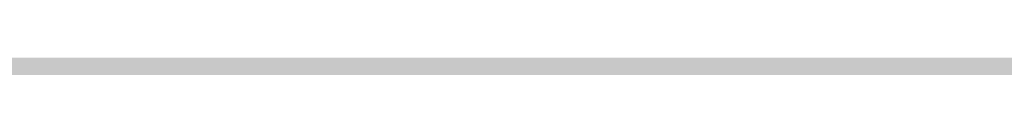
# Model space of a CAD drawing. Units: millimetres. Extents: x 0 to 2267, y 0 to 1823.
# Tile 206 of 256: x 1841.442 to 1842.748, y 1127.404 to 1127.414. Entities that reach past the tile are written whole.
import ezdxf

# ---------------------------------------------------------------- set-up
doc = ezdxf.new("R2010")
doc.units = ezdxf.units.MM
doc.header["$MEASUREMENT"] = 0
doc.layers.add('M-DIMS', color=2, linetype='Continuous', lineweight=25)
doc.layers.add('M-HATC', color=252, linetype='Continuous', lineweight=18)
doc.styles.get("Standard").update_dxf_attribs({"font": 'arial.ttf'})
doc.dimstyles.get("Standard").update_dxf_attribs({"dimtxt": 7, "dimasz": 4, "dimexe": 0.18, "dimexo": 0.0625, "dimgap": 0.09, "dimtad": 0, "dimdec": 0, "dimzin": 0, "dimdsep": 46, "dimtxsty": 'Standard', "dimcen": 0.09, "dimadec": 0, "dimazin": 0, "dimtfac": 1, "dimtdec": 0, "dimtofl": 0, "dimtmove": 0, "dimatfit": 3, "dimfxl": 1, "dimtolj": 1, "dimtzin": 0, "dimarcsym": 0})

# ---------------------------------------------------------------- blocks, each defined once
blk = doc.blocks.new('*D1')
at = {"layer": 'Defpoints', "color": 0, "transparency": 16777216}
for p in [(1593.4289, 1127.4171), (1843.4289, 1127.4171), (1843.4289, 955.6278)]:
    blk.add_point(p, dxfattribs=at)
at = {"layer": 'M-DIMS', "color": 0, "lineweight": -2, "transparency": 16777216}
for p, q in [((1593.4289, 1127.3546), (1593.4289, 955.4478)), ((1843.4289, 1127.3546), (1843.4289, 955.4478)), ((1597.4289, 955.6278), (1710.5582, 955.6278)), ((1839.4289, 955.6278), (1726.2996, 955.6278))]:
    blk.add_line(p, q, dxfattribs=at)
at = {"layer": 'M-DIMS', "color": 0, "transparency": 16777216}
for points in [[(1597.4289, 956.2944), (1597.4289, 954.9611), (1593.4289, 955.6278)], [(1839.4289, 956.2944), (1839.4289, 954.9611), (1843.4289, 955.6278)]]:
    blk.add_solid(points, dxfattribs=at)
at = {"layer": 'M-DIMS', "color": 0, "transparency": 16777216, "insert": (1718.4289, 955.6278), "char_height": 7, "attachment_point": 5}
blk.add_mtext('\\A1;250', dxfattribs=at)

msp = doc.modelspace()

# ---------------------------------------------------------------- hatches: boundary and pattern name
at = {"layer": 'M-HATC'}
h = msp.add_hatch(color=256, dxfattribs=at)
h.dxf.hatch_style = 1
h.paths.add_polyline_path([(2055.771, 1603.062), (1381.0868, 1603.062), (1381.0868, 1598.062), (2055.771, 1598.062)])
h.paths.add_polyline_path([(2055.771, 1598.062), (1381.0868, 1598.062), (1381.0868, 1593.062), (2055.771, 1593.062)])
h.paths.add_polyline_path([(2051.3074, 1536.7609), (1385.5504, 1536.7609), (1385.5504, 1526.7609), (1387.5504, 1526.7609), (1388.5366, 1525.0528), (1385.3319, 1521.2335), (1385.3319, 1521.2226), (2050.2542, 1522.7491), (2048.3212, 1525.0528), (2049.3074, 1526.7609), (2051.3074, 1526.7609)])
edge = h.paths.add_edge_path()
edge.add_arc((1847.5345, 1379.1492), 135, 222.603061, 222.890851, ccw=False)
edge.add_line((1748.1663, 1287.7656), (1683.0921, 1287.7656))
edge.add_arc((1583.7239, 1379.1492), 135, 317.109149, 317.396939, ccw=False)
edge.add_arc((1678.9686, 1290.6707), 5, 222.8909, 317.1091, ccw=False)
edge.add_arc((1774.2133, 1379.1492), 135, 222.603061, 222.890851, ccw=False)
edge.add_line((1674.8451, 1287.7656), (1609.7709, 1287.7656))
edge.add_arc((1510.4027, 1379.1492), 135, 317.109149, 317.396939, ccw=False)
edge.add_arc((1605.6474, 1290.6707), 5, 222.8909, 317.1091, ccw=False)
edge.add_arc((1700.8921, 1379.1492), 135, 222.603061, 222.890851, ccw=False)
edge.add_line((1601.5239, 1287.7656), (1536.4497, 1287.7656))
edge.add_arc((1437.0815, 1379.1492), 135, 317.109149, 317.396939, ccw=False)
edge.add_arc((1532.3262, 1290.6707), 5, 222.8909, 317.1091, ccw=False)
edge.add_arc((1627.5709, 1379.1492), 135, 222.603061, 222.890851, ccw=False)
edge.add_line((1528.2027, 1287.7656), (1505.9289, 1287.7656))
edge.add_spline(control_points=[(1505.9289, 1287.7656), (1504.2622, 1287.7656), (1504.2622, 1282.7656), (1505.9289, 1282.7656)], knot_values=[0, 0, 0, 0, 5, 5, 5, 5], degree=3, periodic=0)
edge.add_line((1505.9289, 1282.7656), (1930.9289, 1282.7656))
edge.add_spline(control_points=[(1930.9289, 1282.7656), (1932.5956, 1282.7656), (1932.5956, 1287.7656), (1930.9289, 1287.7656)], knot_values=[0, 0, 0, 0, 5, 5, 5, 5], degree=3, periodic=0)
edge.add_line((1930.9289, 1287.7656), (1903.0557, 1287.7656))
edge.add_arc((1803.6875, 1379.1492), 135, 317.109149, 317.396939, ccw=False)
edge.add_arc((1898.9322, 1290.6707), 5, 222.8909, 317.1091, ccw=False)
edge.add_arc((1994.1769, 1379.1492), 135, 222.603061, 222.890851, ccw=False)
edge.add_line((1894.8087, 1287.7656), (1829.7345, 1287.7656))
edge.add_arc((1730.3663, 1379.1492), 135, 317.109149, 317.396939, ccw=False)
edge.add_arc((1825.611, 1290.6707), 5, 222.8909, 317.1091, ccw=False)
edge.add_arc((1920.8557, 1379.1492), 135, 222.603061, 222.890851, ccw=False)
edge.add_line((1821.4875, 1287.7656), (1756.4133, 1287.7656))
edge.add_arc((1657.0451, 1379.1492), 135, 317.109149, 317.396939, ccw=False)
edge.add_arc((1752.2898, 1290.6707), 5, 222.8909, 317.1091, ccw=False)
edge = h.paths.add_edge_path()
edge.add_spline(control_points=[(1843.4289, 1227.2475), (1845.0956, 1227.2475), (1845.0956, 1232.2475), (1843.4289, 1232.2475)], knot_values=[0, 0, 0, 0, 5, 5, 5, 5], degree=3, periodic=0)
edge.add_line((1843.4289, 1232.2475), (1593.4289, 1232.2475))
edge.add_spline(control_points=[(1593.4289, 1232.2475), (1591.7622, 1232.2475), (1591.7622, 1227.2475), (1593.4289, 1227.2475)], knot_values=[0, 0, 0, 0, 5, 5, 5, 5], degree=3, periodic=0)
edge.add_line((1593.4289, 1227.2475), (1843.4289, 1227.2475))
h.paths.add_polyline_path([(1905.9289, 1127.4171), (1530.9289, 1127.4171, 0.414214), (1520.9289, 1117.4171), (1530.9289, 1117.4171), (1915.9289, 1117.4171, 0.414214)])
edge = h.paths.add_edge_path()
edge.add_arc((1397.0858, 1498.4078), 12.7299, 90.78215, 190.87871, ccw=False)
edge.add_line((1396.912, 1511.1365), (1428.0097, 1511.3488))
edge.add_line((1428.0097, 1511.3488), (1433.0097, 1511.3488))
edge.add_line((1433.0097, 1511.3488), (1434.439, 1511.3488))
edge.add_arc((1419.474, 1498.0804), 20, 41.561, 74.08211)
edge.add_line((1424.9592, 1517.3135), (1399.9351, 1517.2561))
edge.add_spline(control_points=[(1399.9307, 1517.2561), (1399.884, 1517.2131), (1399.8328, 1517.1689), (1399.7774, 1517.1236)], knot_values=[11.567499, 11.567499, 11.567499, 11.567499, 11.814249, 11.814249, 11.814249, 11.814249], degree=3, periodic=0)
edge.add_spline(control_points=[(1399.6328, 1517.0099), (1399.5831, 1516.9721), (1399.5307, 1516.9338), (1399.4759, 1516.8947)], knot_values=[11.167718, 11.167718, 11.167718, 11.167718, 11.365188, 11.365188, 11.365188, 11.365188], degree=3, periodic=0)
edge.add_spline(control_points=[(1399.3398, 1516.8001), (1399.1514, 1516.6719), (1398.9384, 1516.5377), (1398.704, 1516.3994)], knot_values=[10.376405, 10.376405, 10.376405, 10.376405, 11.00994, 11.00994, 11.00994, 11.00994], degree=3, periodic=0)
edge.add_spline(control_points=[(1398.6572, 1516.3719), (1398.5789, 1516.326), (1398.4983, 1516.2797), (1398.4155, 1516.2331)], knot_values=[10.125175, 10.125175, 10.125175, 10.125175, 10.334406, 10.334406, 10.334406, 10.334406], degree=3, periodic=0)
edge.add_spline(control_points=[(1398.2642, 1516.1487), (1398.196, 1516.1111), (1398.1263, 1516.0732), (1398.0555, 1516.0351)], knot_values=[9.832246, 9.832246, 9.832246, 9.832246, 9.999658, 9.999658, 9.999658, 9.999658], degree=3, periodic=0)
edge.add_spline(control_points=[(1397.9987, 1516.0048), (1397.7312, 1515.8621), (1397.446, 1515.7171), (1397.1466, 1515.5714)], knot_values=[9.161808, 9.161808, 9.161808, 9.161808, 9.787769, 9.787769, 9.787769, 9.787769], degree=3, periodic=0)
edge.add_spline(control_points=[(1397.1466, 1515.5714), (1396.8418, 1515.423), (1396.5222, 1515.274), (1396.1914, 1515.1262)], knot_values=[8.524455, 8.524455, 8.524455, 8.524455, 9.161808, 9.161808, 9.161808, 9.161808], degree=3, periodic=0)
edge.add_spline(control_points=[(1396.0777, 1515.0756), (1395.9854, 1515.0348), (1395.8922, 1514.994), (1395.7983, 1514.9534)], knot_values=[8.275193, 8.275193, 8.275193, 8.275193, 8.451726, 8.451726, 8.451726, 8.451726], degree=3, periodic=0)
edge.add_spline(control_points=[(1395.6018, 1514.8691), (1395.4997, 1514.8257), (1395.3968, 1514.7824), (1395.2932, 1514.7394)], knot_values=[7.962917, 7.962917, 7.962917, 7.962917, 8.152764, 8.152764, 8.152764, 8.152764], degree=3, periodic=0)
edge.add_spline(control_points=[(1395.2116, 1514.7057), (1394.8278, 1514.5475), (1394.4345, 1514.3929), (1394.0364, 1514.2442)], knot_values=[7.21254, 7.21254, 7.21254, 7.21254, 7.913148, 7.913148, 7.913148, 7.913148], degree=3, periodic=0)
edge.add_spline(control_points=[(1394.0364, 1514.2442), (1393.7076, 1514.1214), (1393.3754, 1514.0027), (1393.0427, 1513.8895)], knot_values=[6.633733, 6.633733, 6.633733, 6.633733, 7.21254, 7.21254, 7.21254, 7.21254], degree=3, periodic=0)
edge.add_spline(control_points=[(1392.8214, 1513.815), (1392.7198, 1513.7812), (1392.6181, 1513.7479), (1392.5166, 1513.7152)], knot_values=[6.328796, 6.328796, 6.328796, 6.328796, 6.505493, 6.505493, 6.505493, 6.505493], degree=3, periodic=0)
edge.add_spline(control_points=[(1392.5166, 1513.7152), (1392.3187, 1513.6515), (1392.1212, 1513.59), (1391.9244, 1513.531)], knot_values=[5.984605, 5.984605, 5.984605, 5.984605, 6.328796, 6.328796, 6.328796, 6.328796], degree=3, periodic=0)
edge.add_spline(control_points=[(1391.7915, 1513.4915), (1391.3122, 1513.3501), (1390.8384, 1513.2239), (1390.3784, 1513.1171)], knot_values=[5.066697, 5.066697, 5.066697, 5.066697, 5.907055, 5.907055, 5.907055, 5.907055], degree=3, periodic=0)
edge.add_spline(control_points=[(1390.3784, 1513.1171), (1390.1797, 1513.071), (1389.9836, 1513.0284), (1389.7907, 1512.9899)], knot_values=[4.70367, 4.70367, 4.70367, 4.70367, 5.066695, 5.066695, 5.066695, 5.066695], degree=3, periodic=0)
edge.add_spline(control_points=[(1389.422, 1512.9204), (1389.2459, 1512.8892), (1389.0729, 1512.8617), (1388.9036, 1512.8381)], knot_values=[4.130571, 4.130571, 4.130571, 4.130571, 4.469816, 4.469816, 4.469816, 4.469816], degree=3, periodic=0)
edge.add_spline(control_points=[(1388.9036, 1512.8381), (1388.591, 1512.7946), (1388.2911, 1512.7644), (1388.0071, 1512.7494)], knot_values=[3.504031, 3.504031, 3.504031, 3.504031, 4.130571, 4.130571, 4.130571, 4.130571], degree=3, periodic=0)
edge.add_spline(control_points=[(1387.9356, 1512.7459), (1387.8538, 1512.7423), (1387.7733, 1512.74), (1387.6944, 1512.739)], knot_values=[3.268866, 3.268866, 3.268866, 3.268866, 3.451164, 3.451164, 3.451164, 3.451164], degree=3, periodic=0)
edge.add_spline(control_points=[(1387.3351, 1512.7443), (1387.2076, 1512.7499), (1387.0847, 1512.7597), (1386.967, 1512.7739)], knot_values=[2.670686, 2.670686, 2.670686, 2.670686, 2.984, 2.984, 2.984, 2.984], degree=3, periodic=0)
edge.add_spline(control_points=[(1386.8327, 1512.7922), (1386.8209, 1512.7941), (1386.8092, 1512.7959), (1386.7975, 1512.7979)], knot_values=[2.516981, 2.516981, 2.516981, 2.516981, 2.549528, 2.549528, 2.549528, 2.549528], degree=3, periodic=0)
edge.add_spline(control_points=[(1386.4526, 1512.8735), (1386.4257, 1512.881), (1386.3993, 1512.889), (1386.3733, 1512.8972)], knot_values=[2.095869, 2.095869, 2.095869, 2.095869, 2.17941, 2.17941, 2.17941, 2.17941], degree=3, periodic=0)
edge.add_spline(control_points=[(1386.0691, 1513.0189), (1386.0634, 1513.0217), (1386.0577, 1513.0246), (1386.052, 1513.0275)], knot_values=[1.72453, 1.72453, 1.72453, 1.72453, 1.745933, 1.745933, 1.745933, 1.745933], degree=3, periodic=0)
edge.add_arc((1399.474, 1498.0804), 20, 131.82432, 180)
edge.add_arc((1630.3336, 1505.5484), 250.9708, 181.705176, 236.427975)
edge.add_arc((1605.3399, 1483.3044), 218.7822, 238.660829, 243.34961)
edge.add_arc((1647.0911, 1510.3592), 262.8986, 183.129836, 237.853442, ccw=False)
h.paths.add_polyline_path([(1406.5369, 1391.9644, 0.149382), (1491.5506, 1296.4418, -0.129517)], flags=17)
edge = h.paths.add_edge_path()
edge.add_arc((2037.3838, 1498.0804), 20, 0, 48.26587)
edge.add_spline(control_points=[(2050.6973, 1513.0052), (2050.6512, 1512.9847), (2050.6034, 1512.9655), (2050.5539, 1512.9477)], knot_values=[1.835652, 1.835652, 1.835652, 1.835652, 2.000781, 2.000781, 2.000781, 2.000781], degree=3, periodic=0)
edge.add_spline(control_points=[(2050.4616, 1512.9166), (2050.479, 1512.9221), (2050.4963, 1512.9277), (2050.5133, 1512.9335)], knot_values=[2.045477, 2.045477, 2.045477, 2.045477, 2.101389, 2.101389, 2.101389, 2.101389], degree=3, periodic=0)
edge.add_spline(control_points=[(2050.129, 1512.8342), (2050.1984, 1512.8473), (2050.2657, 1512.8623), (2050.3308, 1512.8792)], knot_values=[2.237629, 2.237629, 2.237629, 2.237629, 2.435841, 2.435841, 2.435841, 2.435841], degree=3, periodic=0)
edge.add_spline(control_points=[(2050.0946, 1512.8278), (2050.1061, 1512.8299), (2050.1176, 1512.832), (2050.129, 1512.8342)], knot_values=[2.435841, 2.435841, 2.435841, 2.435841, 2.468321, 2.468321, 2.468321, 2.468321], degree=3, periodic=0)
edge.add_spline(control_points=[(2049.7843, 1512.7851), (2049.8552, 1512.7922), (2049.9243, 1512.8008), (2049.9917, 1512.8109)], knot_values=[2.563852, 2.563852, 2.563852, 2.563852, 2.748541, 2.748541, 2.748541, 2.748541], degree=3, periodic=0)
edge.add_spline(control_points=[(2049.4052, 1512.7617), (2049.5364, 1512.7653), (2049.6629, 1512.773), (2049.7843, 1512.7851)], knot_values=[2.748541, 2.748541, 2.748541, 2.748541, 3.064882, 3.064882, 3.064882, 3.064882], degree=3, periodic=0)
edge.add_spline(control_points=[(2049.1698, 1512.7597), (2049.2336, 1512.7591), (2049.2965, 1512.7594), (2049.3584, 1512.7606)], knot_values=[3.102309, 3.102309, 3.102309, 3.102309, 3.2503, 3.2503, 3.2503, 3.2503], degree=3, periodic=0)
edge.add_spline(control_points=[(2048.8573, 1512.7691), (2048.9638, 1512.7638), (2049.068, 1512.7606), (2049.1698, 1512.7597)], knot_values=[3.2503, 3.2503, 3.2503, 3.2503, 3.486069, 3.486069, 3.486069, 3.486069], degree=3, periodic=0)
edge.add_spline(control_points=[(2048.6924, 1512.7789), (2048.3729, 1512.8009), (2048.0345, 1512.8411), (2047.6817, 1512.897)], knot_values=[3.606429, 3.606429, 3.606429, 3.606429, 4.2989, 4.2989, 4.2989, 4.2989], degree=3, periodic=0)
edge.add_spline(control_points=[(2047.6817, 1512.897), (2047.5458, 1512.9185), (2047.4077, 1512.9424), (2047.2678, 1512.9685)], knot_values=[4.2989, 4.2989, 4.2989, 4.2989, 4.565769, 4.565769, 4.565769, 4.565769], degree=3, periodic=0)
edge.add_spline(control_points=[(2047.2678, 1512.9685), (2047.1449, 1512.9914), (2047.0207, 1513.016), (2046.8951, 1513.0422)], knot_values=[4.565769, 4.565769, 4.565769, 4.565769, 4.799971, 4.799971, 4.799971, 4.799971], degree=3, periodic=0)
edge.add_spline(control_points=[(2046.8951, 1513.0422), (2046.5286, 1513.1188), (2046.1513, 1513.209), (2045.7676, 1513.3107)], knot_values=[4.799971, 4.799971, 4.799971, 4.799971, 5.483718, 5.483718, 5.483718, 5.483718], degree=3, periodic=0)
edge.add_spline(control_points=[(2045.7676, 1513.3107), (2045.3724, 1513.4154), (2044.9704, 1513.5322), (2044.5662, 1513.6588)], knot_values=[5.483718, 5.483718, 5.483718, 5.483718, 6.187866, 6.187866, 6.187866, 6.187866], degree=3, periodic=0)
edge.add_spline(control_points=[(2044.5662, 1513.6588), (2044.4149, 1513.7061), (2044.2633, 1513.7549), (2044.1116, 1513.8048)], knot_values=[6.187866, 6.187866, 6.187866, 6.187866, 6.451551, 6.451551, 6.451551, 6.451551], degree=3, periodic=0)
edge.add_spline(control_points=[(2044.1116, 1513.8048), (2043.9967, 1513.8427), (2043.8817, 1513.8813), (2043.7668, 1513.9205)], knot_values=[6.451551, 6.451551, 6.451551, 6.451551, 6.651434, 6.651434, 6.651434, 6.651434], degree=3, periodic=0)
edge.add_spline(control_points=[(2043.7668, 1513.9205), (2043.3716, 1514.0554), (2042.9774, 1514.1979), (2042.5886, 1514.3458)], knot_values=[6.651434, 6.651434, 6.651434, 6.651434, 7.338879, 7.338879, 7.338879, 7.338879], degree=3, periodic=0)
edge.add_spline(control_points=[(2042.5886, 1514.3458), (2042.1643, 1514.5071), (2041.7465, 1514.6749), (2041.3409, 1514.846)], knot_values=[7.338879, 7.338879, 7.338879, 7.338879, 8.089209, 8.089209, 8.089209, 8.089209], degree=3, periodic=0)
edge.add_spline(control_points=[(2041.3409, 1514.846), (2041.1028, 1514.9465), (2040.869, 1515.0481), (2040.6405, 1515.1502)], knot_values=[8.089209, 8.089209, 8.089209, 8.089209, 8.529587, 8.529587, 8.529587, 8.529587], degree=3, periodic=0)
edge.add_spline(control_points=[(2040.51, 1515.2089), (2040.0824, 1515.4022), (2039.6747, 1515.5971), (2039.295, 1515.7894)], knot_values=[8.613818, 8.613818, 8.613818, 8.613818, 9.44571, 9.44571, 9.44571, 9.44571], degree=3, periodic=0)
edge.add_spline(control_points=[(2039.295, 1515.7894), (2039.0618, 1515.9075), (2038.8391, 1516.0246), (2038.6288, 1516.1398)], knot_values=[9.44571, 9.44571, 9.44571, 9.44571, 9.956404, 9.956404, 9.956404, 9.956404], degree=3, periodic=0)
edge.add_spline(control_points=[(2038.6288, 1516.1398), (2038.5187, 1516.2001), (2038.4121, 1516.2598), (2038.309, 1516.3189)], knot_values=[9.956404, 9.956404, 9.956404, 9.956404, 10.223542, 10.223542, 10.223542, 10.223542], degree=3, periodic=0)
edge.add_spline(control_points=[(2038.309, 1516.3189), (2038.2138, 1516.3735), (2038.1216, 1516.4276), (2038.0328, 1516.481)], knot_values=[10.223542, 10.223542, 10.223542, 10.223542, 10.47051, 10.47051, 10.47051, 10.47051], degree=3, periodic=0)
edge.add_spline(control_points=[(2038.0328, 1516.481), (2037.7855, 1516.6296), (2037.5639, 1516.773), (2037.3722, 1516.909)], knot_values=[10.47051, 10.47051, 10.47051, 10.47051, 11.15767, 11.15767, 11.15767, 11.15767], degree=3, periodic=0)
edge.add_spline(control_points=[(2037.3722, 1516.909), (2037.2789, 1516.9752), (2037.1927, 1517.0396), (2037.1142, 1517.102)], knot_values=[11.15767, 11.15767, 11.15767, 11.15767, 11.49227, 11.49227, 11.49227, 11.49227], degree=3, periodic=0)
edge.add_spline(control_points=[(2036.8564, 1517.3259), (2036.9148, 1517.2692), (2036.9814, 1517.2103), (2037.0557, 1517.1492)], knot_values=[11.577341, 11.577341, 11.577341, 11.577341, 11.91035, 11.91035, 11.91035, 11.91035], degree=3, periodic=0)
edge.add_spline(control_points=[(2036.8074, 1517.3748), (2036.823, 1517.3587), (2036.8393, 1517.3424), (2036.8564, 1517.3259)], knot_values=[11.91035, 11.91035, 11.91035, 11.91035, 12.007402, 12.007402, 12.007402, 12.007402], degree=3, periodic=0)
edge.add_spline(control_points=[(2036.7017, 1517.494), (2036.7104, 1517.483), (2036.7196, 1517.4719), (2036.7291, 1517.4606)], knot_values=[12.184155, 12.184155, 12.184155, 12.184155, 12.255409, 12.255409, 12.255409, 12.255409], degree=3, periodic=0)
edge.add_spline(control_points=[(2036.6159, 1517.6205), (2036.62, 1517.613), (2036.6243, 1517.6055), (2036.6289, 1517.5979)], knot_values=[12.487913, 12.487913, 12.487913, 12.487913, 12.541035, 12.541035, 12.541035, 12.541035], degree=3, periodic=0)
edge.add_spline(control_points=[(2036.5635, 1517.786), (2036.5637, 1517.7794), (2036.5642, 1517.7726), (2036.565, 1517.7658)], knot_values=[12.911761, 12.911761, 12.911761, 12.911761, 12.968286, 12.968286, 12.968286, 12.968286], degree=3, periodic=0)
edge.add_spline(control_points=[(2036.6166, 1517.9304), (2036.6125, 1517.9259), (2036.6086, 1517.9212), (2036.6049, 1517.9165)], knot_values=[13.382527, 13.382527, 13.382527, 13.382527, 13.433791, 13.433791, 13.433791, 13.433791], degree=3, periodic=0)
edge.add_spline(control_points=[(2036.749, 1518.017), (2036.7361, 1518.0116), (2036.7239, 1518.006), (2036.7124, 1518.0002)], knot_values=[13.726299, 13.726299, 13.726299, 13.726299, 13.809928, 13.809928, 13.809928, 13.809928], degree=3, periodic=0)
edge.add_spline(control_points=[(2036.8604, 1518.0528), (2036.8386, 1518.0474), (2036.8181, 1518.0416), (2036.7988, 1518.0353)], knot_values=[13.910887, 13.910887, 13.910887, 13.910887, 14.02153, 14.02153, 14.02153, 14.02153], degree=3, periodic=0)
edge.add_line((2036.9639, 1518.0804), (2032.3838, 1518.0804))
edge.add_line((2032.3838, 1518.0804), (2027.3838, 1518.0804))
edge.add_line((2027.3838, 1518.0804), (2022.3838, 1518.0804))
edge.add_line((2022.3838, 1518.0804), (2017.3838, 1518.0804))
edge.add_arc((2017.3838, 1498.0804), 20, 90, 138.439)
edge.add_line((2002.4188, 1511.3488), (2003.8481, 1511.3488))
edge.add_line((2003.8481, 1511.3488), (2008.8481, 1511.3488))
edge.add_line((2008.8481, 1511.3488), (2039.772, 1511.1377))
edge.add_arc((2039.772, 1498.4078), 12.7299, -10.87871, 90, ccw=False)
edge.add_arc((1789.7668, 1510.3592), 262.8986, 302.146558, 356.870164, ccw=False)
edge.add_arc((1831.5179, 1483.3044), 218.7822, 296.65039, 301.339171)
edge.add_arc((1806.5242, 1505.5484), 250.9708, 303.572025, 358.294824)
h.paths.add_polyline_path([(2030.321, 1391.9644, -0.129517), (1945.3072, 1296.4418, 0.149382)], flags=17)
edge = h.paths.add_edge_path()
edge.add_spline(control_points=[(2037.2464, 1518.0821), (2037.2898, 1518.081), (2037.3355, 1518.0804), (2037.3838, 1518.0804)], knot_values=[0.000012, 0.000012, 0.000012, 0.000012, 0.144754, 0.144754, 0.144754, 0.144754], degree=3, periodic=0)
edge.add_line((2037.3357, 1518.0804), (2037.0096, 1518.0804))
edge.add_spline(control_points=[(2037.0096, 1518.0804), (2036.9822, 1518.0768), (2036.956, 1518.0727), (2036.9312, 1518.0681)], knot_values=[14.13465, 14.13465, 14.13465, 14.13465, 14.247197, 14.247197, 14.247197, 14.247197], degree=3, periodic=0)
edge.add_spline(control_points=[(2036.9312, 1518.0681), (2036.9276, 1518.0674), (2036.9241, 1518.0667), (2036.9205, 1518.0661)], knot_values=[14.118315, 14.118315, 14.118315, 14.118315, 14.13465, 14.13465, 14.13465, 14.13465], degree=3, periodic=0)
edge.add_spline(control_points=[(2036.9205, 1518.0661), (2036.9118, 1518.0644), (2036.9032, 1518.0626), (2036.8948, 1518.0608)], knot_values=[14.078086, 14.078086, 14.078086, 14.078086, 14.118315, 14.118315, 14.118315, 14.118315], degree=3, periodic=0)
edge.add_spline(control_points=[(2036.8948, 1518.0608), (2036.883, 1518.0583), (2036.8716, 1518.0556), (2036.8604, 1518.0528)], knot_values=[14.02153, 14.02153, 14.02153, 14.02153, 14.078086, 14.078086, 14.078086, 14.078086], degree=3, periodic=0)
edge.add_spline(control_points=[(2036.8604, 1518.0528), (2036.8386, 1518.0474), (2036.8181, 1518.0416), (2036.7988, 1518.0353)], knot_values=[13.910887, 13.910887, 13.910887, 13.910887, 14.02153, 14.02153, 14.02153, 14.02153], degree=3, periodic=0)
edge.add_spline(control_points=[(2036.7988, 1518.0353), (2036.7981, 1518.035), (2036.7974, 1518.0348), (2036.7967, 1518.0346)], knot_values=[13.906906, 13.906906, 13.906906, 13.906906, 13.910887, 13.910887, 13.910887, 13.910887], degree=3, periodic=0)
edge.add_spline(control_points=[(2036.7967, 1518.0346), (2036.7882, 1518.0318), (2036.7799, 1518.0289), (2036.7719, 1518.0259)], knot_values=[13.857826, 13.857826, 13.857826, 13.857826, 13.906906, 13.906906, 13.906906, 13.906906], degree=3, periodic=0)
edge.add_spline(control_points=[(2036.7719, 1518.0259), (2036.764, 1518.023), (2036.7564, 1518.02), (2036.749, 1518.017)], knot_values=[13.809928, 13.809928, 13.809928, 13.809928, 13.857826, 13.857826, 13.857826, 13.857826], degree=3, periodic=0)
edge.add_spline(control_points=[(2036.749, 1518.017), (2036.7361, 1518.0116), (2036.7239, 1518.006), (2036.7124, 1518.0002)], knot_values=[13.726299, 13.726299, 13.726299, 13.726299, 13.809928, 13.809928, 13.809928, 13.809928], degree=3, periodic=0)
edge.add_spline(control_points=[(2036.7124, 1518.0002), (2036.7121, 1518), (2036.7118, 1517.9999), (2036.7115, 1517.9997)], knot_values=[13.723993, 13.723993, 13.723993, 13.723993, 13.726299, 13.726299, 13.726299, 13.726299], degree=3, periodic=0)
edge.add_spline(control_points=[(2036.7115, 1517.9997), (2036.7063, 1517.9971), (2036.7013, 1517.9944), (2036.6965, 1517.9917)], knot_values=[13.686536, 13.686536, 13.686536, 13.686536, 13.723993, 13.723993, 13.723993, 13.723993], degree=3, periodic=0)
edge.add_spline(control_points=[(2036.6965, 1517.9917), (2036.6919, 1517.9891), (2036.6874, 1517.9865), (2036.6831, 1517.9839)], knot_values=[13.651251, 13.651251, 13.651251, 13.651251, 13.686536, 13.686536, 13.686536, 13.686536], degree=3, periodic=0)
edge.add_spline(control_points=[(2036.6831, 1517.9839), (2036.6764, 1517.9798), (2036.67, 1517.9757), (2036.6639, 1517.9714)], knot_values=[13.596804, 13.596804, 13.596804, 13.596804, 13.651251, 13.651251, 13.651251, 13.651251], degree=3, periodic=0)
edge.add_spline(control_points=[(2036.6639, 1517.9714), (2036.6636, 1517.9712), (2036.6633, 1517.9709), (2036.6629, 1517.9707)], knot_values=[13.593956, 13.593956, 13.593956, 13.593956, 13.596804, 13.596804, 13.596804, 13.596804], degree=3, periodic=0)
edge.add_spline(control_points=[(2036.6629, 1517.9707), (2036.6603, 1517.9689), (2036.6577, 1517.967), (2036.6552, 1517.9651)], knot_values=[13.570322, 13.570322, 13.570322, 13.570322, 13.593956, 13.593956, 13.593956, 13.593956], degree=3, periodic=0)
edge.add_spline(control_points=[(2036.6552, 1517.9651), (2036.6525, 1517.9631), (2036.6499, 1517.9611), (2036.6474, 1517.9591)], knot_values=[13.545477, 13.545477, 13.545477, 13.545477, 13.570322, 13.570322, 13.570322, 13.570322], degree=3, periodic=0)
edge.add_spline(control_points=[(2036.6474, 1517.9591), (2036.6472, 1517.9589), (2036.6471, 1517.9588), (2036.6469, 1517.9587)], knot_values=[13.543931, 13.543931, 13.543931, 13.543931, 13.545477, 13.545477, 13.545477, 13.545477], degree=3, periodic=0)
edge.add_spline(control_points=[(2036.6469, 1517.9587), (2036.6412, 1517.9541), (2036.6358, 1517.9494), (2036.6307, 1517.9447)], knot_values=[13.488237, 13.488237, 13.488237, 13.488237, 13.543931, 13.543931, 13.543931, 13.543931], degree=3, periodic=0)
edge.add_spline(control_points=[(2036.6307, 1517.9447), (2036.6282, 1517.9423), (2036.6257, 1517.9399), (2036.6233, 1517.9374)], knot_values=[13.460307, 13.460307, 13.460307, 13.460307, 13.488237, 13.488237, 13.488237, 13.488237], degree=3, periodic=0)
edge.add_spline(control_points=[(2036.6233, 1517.9374), (2036.6215, 1517.9356), (2036.6198, 1517.9338), (2036.6181, 1517.932)], knot_values=[13.439712, 13.439712, 13.439712, 13.439712, 13.460307, 13.460307, 13.460307, 13.460307], degree=3, periodic=0)
edge.add_spline(control_points=[(2036.6181, 1517.932), (2036.6176, 1517.9315), (2036.6171, 1517.9309), (2036.6166, 1517.9304)], knot_values=[13.433791, 13.433791, 13.433791, 13.433791, 13.439712, 13.439712, 13.439712, 13.439712], degree=3, periodic=0)
edge.add_spline(control_points=[(2036.6166, 1517.9304), (2036.6125, 1517.9259), (2036.6086, 1517.9212), (2036.6049, 1517.9165)], knot_values=[13.382527, 13.382527, 13.382527, 13.382527, 13.433791, 13.433791, 13.433791, 13.433791], degree=3, periodic=0)
edge.add_spline(control_points=[(2036.6049, 1517.9165), (2036.6026, 1517.9135), (2036.6004, 1517.9104), (2036.5982, 1517.9074)], knot_values=[13.350017, 13.350017, 13.350017, 13.350017, 13.382527, 13.382527, 13.382527, 13.382527], degree=3, periodic=0)
edge.add_spline(control_points=[(2036.5982, 1517.9074), (2036.5972, 1517.9059), (2036.5962, 1517.9043), (2036.5952, 1517.9028)], knot_values=[13.333922, 13.333922, 13.333922, 13.333922, 13.350017, 13.350017, 13.350017, 13.350017], degree=3, periodic=0)
edge.add_spline(control_points=[(2036.5952, 1517.9028), (2036.5945, 1517.9018), (2036.5939, 1517.9009), (2036.5933, 1517.8999)], knot_values=[13.323828, 13.323828, 13.323828, 13.323828, 13.333922, 13.333922, 13.333922, 13.333922], degree=3, periodic=0)
edge.add_spline(control_points=[(2036.5933, 1517.8999), (2036.5905, 1517.8955), (2036.5879, 1517.8909), (2036.5855, 1517.8864)], knot_values=[13.277545, 13.277545, 13.277545, 13.277545, 13.323828, 13.323828, 13.323828, 13.323828], degree=3, periodic=0)
edge.add_spline(control_points=[(2036.5855, 1517.8864), (2036.5836, 1517.8827), (2036.5817, 1517.8789), (2036.5801, 1517.8751)], knot_values=[13.240119, 13.240119, 13.240119, 13.240119, 13.277545, 13.277545, 13.277545, 13.277545], degree=3, periodic=0)
edge.add_spline(control_points=[(2036.5801, 1517.8751), (2036.5795, 1517.8739), (2036.579, 1517.8727), (2036.5785, 1517.8715)], knot_values=[13.228211, 13.228211, 13.228211, 13.228211, 13.240119, 13.240119, 13.240119, 13.240119], degree=3, periodic=0)
edge.add_spline(control_points=[(2036.5785, 1517.8715), (2036.578, 1517.8702), (2036.5774, 1517.869), (2036.5769, 1517.8677)], knot_values=[13.215717, 13.215717, 13.215717, 13.215717, 13.228211, 13.228211, 13.228211, 13.228211], degree=3, periodic=0)
edge.add_spline(control_points=[(2036.5769, 1517.8677), (2036.5755, 1517.864), (2036.5741, 1517.8603), (2036.5729, 1517.8565)], knot_values=[13.179847, 13.179847, 13.179847, 13.179847, 13.215717, 13.215717, 13.215717, 13.215717], degree=3, periodic=0)
edge.add_spline(control_points=[(2036.5729, 1517.8565), (2036.5713, 1517.8515), (2036.5699, 1517.8464), (2036.5687, 1517.8413)], knot_values=[13.132017, 13.132017, 13.132017, 13.132017, 13.179847, 13.179847, 13.179847, 13.179847], degree=3, periodic=0)
edge.add_spline(control_points=[(2036.5687, 1517.8413), (2036.5684, 1517.8402), (2036.5682, 1517.8392), (2036.568, 1517.8382)], knot_values=[13.122482, 13.122482, 13.122482, 13.122482, 13.132017, 13.132017, 13.132017, 13.132017], degree=3, periodic=0)
edge.add_spline(control_points=[(2036.568, 1517.8382), (2036.5676, 1517.8363), (2036.5672, 1517.8345), (2036.5669, 1517.8327)], knot_values=[13.105592, 13.105592, 13.105592, 13.105592, 13.122482, 13.122482, 13.122482, 13.122482], degree=3, periodic=0)
edge.add_spline(control_points=[(2036.5669, 1517.8327), (2036.5662, 1517.8292), (2036.5657, 1517.8257), (2036.5652, 1517.8222)], knot_values=[13.074063, 13.074063, 13.074063, 13.074063, 13.105592, 13.105592, 13.105592, 13.105592], degree=3, periodic=0)
edge.add_spline(control_points=[(2036.5652, 1517.8222), (2036.5652, 1517.8222), (2036.5652, 1517.8222), (2036.5652, 1517.8222)], knot_values=[13.074043, 13.074043, 13.074043, 13.074043, 13.074063, 13.074063, 13.074063, 13.074063], degree=3, periodic=0)
edge.add_spline(control_points=[(2036.5652, 1517.8222), (2036.5644, 1517.8164), (2036.5639, 1517.8106), (2036.5636, 1517.8046)], knot_values=[13.021884, 13.021884, 13.021884, 13.021884, 13.074043, 13.074043, 13.074043, 13.074043], degree=3, periodic=0)
edge.add_spline(control_points=[(2036.5636, 1517.8046), (2036.5636, 1517.804), (2036.5636, 1517.8034), (2036.5635, 1517.8028)], knot_values=[13.01674, 13.01674, 13.01674, 13.01674, 13.021884, 13.021884, 13.021884, 13.021884], degree=3, periodic=0)
edge.add_spline(control_points=[(2036.5635, 1517.8028), (2036.5634, 1517.8005), (2036.5634, 1517.7982), (2036.5634, 1517.7958)], knot_values=[12.996438, 12.996438, 12.996438, 12.996438, 13.01674, 13.01674, 13.01674, 13.01674], degree=3, periodic=0)
edge.add_spline(control_points=[(2036.5634, 1517.7958), (2036.5633, 1517.7926), (2036.5634, 1517.7893), (2036.5635, 1517.786)], knot_values=[12.968286, 12.968286, 12.968286, 12.968286, 12.996438, 12.996438, 12.996438, 12.996438], degree=3, periodic=0)
edge.add_spline(control_points=[(2036.5635, 1517.786), (2036.5637, 1517.7794), (2036.5642, 1517.7726), (2036.565, 1517.7658)], knot_values=[12.911761, 12.911761, 12.911761, 12.911761, 12.968286, 12.968286, 12.968286, 12.968286], degree=3, periodic=0)
edge.add_spline(control_points=[(2036.565, 1517.7658), (2036.565, 1517.7657), (2036.565, 1517.7656), (2036.565, 1517.7656)], knot_values=[12.911017, 12.911017, 12.911017, 12.911017, 12.911761, 12.911761, 12.911761, 12.911761], degree=3, periodic=0)
edge.add_spline(control_points=[(2036.565, 1517.7656), (2036.5654, 1517.7625), (2036.5658, 1517.7593), (2036.5663, 1517.7562)], knot_values=[12.88528, 12.88528, 12.88528, 12.88528, 12.911017, 12.911017, 12.911017, 12.911017], degree=3, periodic=0)
edge.add_spline(control_points=[(2036.5663, 1517.7562), (2036.5667, 1517.7534), (2036.5672, 1517.7506), (2036.5677, 1517.7478)], knot_values=[12.862519, 12.862519, 12.862519, 12.862519, 12.88528, 12.88528, 12.88528, 12.88528], degree=3, periodic=0)
edge.add_spline(control_points=[(2036.5677, 1517.7478), (2036.5678, 1517.7474), (2036.5679, 1517.7469), (2036.568, 1517.7465)], knot_values=[12.858885, 12.858885, 12.858885, 12.858885, 12.862519, 12.862519, 12.862519, 12.862519], degree=3, periodic=0)
edge.add_spline(control_points=[(2036.568, 1517.7465), (2036.5692, 1517.7399), (2036.5707, 1517.7332), (2036.5724, 1517.7264)], knot_values=[12.8053, 12.8053, 12.8053, 12.8053, 12.858885, 12.858885, 12.858885, 12.858885], degree=3, periodic=0)
edge.add_spline(control_points=[(2036.5724, 1517.7264), (2036.5734, 1517.7226), (2036.5745, 1517.7187), (2036.5756, 1517.7149)], knot_values=[12.775176, 12.775176, 12.775176, 12.775176, 12.8053, 12.8053, 12.8053, 12.8053], degree=3, periodic=0)
edge.add_spline(control_points=[(2036.5756, 1517.7149), (2036.5763, 1517.7125), (2036.577, 1517.7102), (2036.5778, 1517.7078)], knot_values=[12.756759, 12.756759, 12.756759, 12.756759, 12.775176, 12.775176, 12.775176, 12.775176], degree=3, periodic=0)
edge.add_spline(control_points=[(2036.5778, 1517.7078), (2036.5781, 1517.7067), (2036.5784, 1517.7057), (2036.5787, 1517.7047)], knot_values=[12.748742, 12.748742, 12.748742, 12.748742, 12.756759, 12.756759, 12.756759, 12.756759], degree=3, periodic=0)
edge.add_spline(control_points=[(2036.5787, 1517.7047), (2036.5808, 1517.6983), (2036.5831, 1517.6919), (2036.5856, 1517.6854)], knot_values=[12.69959, 12.69959, 12.69959, 12.69959, 12.748742, 12.748742, 12.748742, 12.748742], degree=3, periodic=0)
edge.add_spline(control_points=[(2036.5856, 1517.6854), (2036.5876, 1517.68), (2036.5898, 1517.6746), (2036.5921, 1517.6692)], knot_values=[12.659038, 12.659038, 12.659038, 12.659038, 12.69959, 12.69959, 12.69959, 12.69959], degree=3, periodic=0)
edge.add_spline(control_points=[(2036.5921, 1517.6692), (2036.594, 1517.6648), (2036.5959, 1517.6605), (2036.5979, 1517.6561)], knot_values=[12.626806, 12.626806, 12.626806, 12.626806, 12.659038, 12.659038, 12.659038, 12.659038], degree=3, periodic=0)
edge.add_spline(control_points=[(2036.5979, 1517.6561), (2036.5984, 1517.6551), (2036.5989, 1517.6541), (2036.5993, 1517.6531)], knot_values=[12.619394, 12.619394, 12.619394, 12.619394, 12.626806, 12.626806, 12.626806, 12.626806], degree=3, periodic=0)
edge.add_spline(control_points=[(2036.5993, 1517.6531), (2036.6043, 1517.6424), (2036.6099, 1517.6315), (2036.6159, 1517.6205)], knot_values=[12.541039, 12.541039, 12.541039, 12.541039, 12.619394, 12.619394, 12.619394, 12.619394], degree=3, periodic=0)
edge.add_spline(control_points=[(2036.6159, 1517.6205), (2036.6159, 1517.6205), (2036.6159, 1517.6205), (2036.6159, 1517.6205)], knot_values=[12.541035, 12.541035, 12.541035, 12.541035, 12.541039, 12.541039, 12.541039, 12.541039], degree=3, periodic=0)
edge.add_spline(control_points=[(2036.6159, 1517.6205), (2036.62, 1517.613), (2036.6243, 1517.6055), (2036.6289, 1517.5979)], knot_values=[12.487913, 12.487913, 12.487913, 12.487913, 12.541035, 12.541035, 12.541035, 12.541035], degree=3, periodic=0)
edge.add_spline(control_points=[(2036.6289, 1517.5979), (2036.6326, 1517.5916), (2036.6365, 1517.5853), (2036.6406, 1517.5789)], knot_values=[12.443982, 12.443982, 12.443982, 12.443982, 12.487913, 12.487913, 12.487913, 12.487913], degree=3, periodic=0)
edge.add_spline(control_points=[(2036.6406, 1517.5789), (2036.6414, 1517.5776), (2036.6423, 1517.5763), (2036.6431, 1517.5749)], knot_values=[12.434996, 12.434996, 12.434996, 12.434996, 12.443982, 12.443982, 12.443982, 12.443982], degree=3, periodic=0)
edge.add_spline(control_points=[(2036.6431, 1517.5749), (2036.6531, 1517.5596), (2036.6639, 1517.5439), (2036.6756, 1517.528)], knot_values=[12.329647, 12.329647, 12.329647, 12.329647, 12.434996, 12.434996, 12.434996, 12.434996], degree=3, periodic=0)
edge.add_spline(control_points=[(2036.6756, 1517.528), (2036.6839, 1517.5168), (2036.6925, 1517.5055), (2036.7017, 1517.494)], knot_values=[12.255409, 12.255409, 12.255409, 12.255409, 12.329647, 12.329647, 12.329647, 12.329647], degree=3, periodic=0)
edge.add_spline(control_points=[(2036.7017, 1517.494), (2036.7104, 1517.483), (2036.7196, 1517.4719), (2036.7291, 1517.4606)], knot_values=[12.184155, 12.184155, 12.184155, 12.184155, 12.255409, 12.255409, 12.255409, 12.255409], degree=3, periodic=0)
edge.add_spline(control_points=[(2036.7291, 1517.4606), (2036.7436, 1517.4435), (2036.759, 1517.4262), (2036.7753, 1517.4085)], knot_values=[12.075961, 12.075961, 12.075961, 12.075961, 12.184155, 12.184155, 12.184155, 12.184155], degree=3, periodic=0)
edge.add_spline(control_points=[(2036.7753, 1517.4085), (2036.7763, 1517.4075), (2036.7773, 1517.4064), (2036.7783, 1517.4054)], knot_values=[12.069502, 12.069502, 12.069502, 12.069502, 12.075961, 12.075961, 12.075961, 12.075961], degree=3, periodic=0)
edge.add_spline(control_points=[(2036.7783, 1517.4054), (2036.7877, 1517.3953), (2036.7974, 1517.385), (2036.8074, 1517.3748)], knot_values=[12.007402, 12.007402, 12.007402, 12.007402, 12.069502, 12.069502, 12.069502, 12.069502], degree=3, periodic=0)
edge.add_spline(control_points=[(2036.8074, 1517.3748), (2036.823, 1517.3587), (2036.8393, 1517.3424), (2036.8564, 1517.3259)], knot_values=[11.91035, 11.91035, 11.91035, 11.91035, 12.007402, 12.007402, 12.007402, 12.007402], degree=3, periodic=0)
edge.add_spline(control_points=[(2036.8564, 1517.3259), (2036.9148, 1517.2692), (2036.9814, 1517.2103), (2037.0557, 1517.1492)], knot_values=[11.577341, 11.577341, 11.577341, 11.577341, 11.91035, 11.91035, 11.91035, 11.91035], degree=3, periodic=0)
edge.add_spline(control_points=[(2037.0557, 1517.1492), (2037.0747, 1517.1336), (2037.0942, 1517.1179), (2037.1142, 1517.102)], knot_values=[11.49227, 11.49227, 11.49227, 11.49227, 11.577341, 11.577341, 11.577341, 11.577341], degree=3, periodic=0)
edge.add_spline(control_points=[(2037.1142, 1517.102), (2037.1927, 1517.0396), (2037.2789, 1516.9752), (2037.3722, 1516.909)], knot_values=[11.15767, 11.15767, 11.15767, 11.15767, 11.49227, 11.49227, 11.49227, 11.49227], degree=3, periodic=0)
edge.add_spline(control_points=[(2037.3722, 1516.909), (2037.5639, 1516.773), (2037.7855, 1516.6296), (2038.0328, 1516.481)], knot_values=[10.47051, 10.47051, 10.47051, 10.47051, 11.15767, 11.15767, 11.15767, 11.15767], degree=3, periodic=0)
edge.add_spline(control_points=[(2038.0328, 1516.481), (2038.1216, 1516.4276), (2038.2138, 1516.3735), (2038.309, 1516.3189)], knot_values=[10.223542, 10.223542, 10.223542, 10.223542, 10.47051, 10.47051, 10.47051, 10.47051], degree=3, periodic=0)
edge.add_spline(control_points=[(2038.309, 1516.3189), (2038.4121, 1516.2598), (2038.5187, 1516.2001), (2038.6288, 1516.1398)], knot_values=[9.956404, 9.956404, 9.956404, 9.956404, 10.223542, 10.223542, 10.223542, 10.223542], degree=3, periodic=0)
edge.add_spline(control_points=[(2038.6288, 1516.1398), (2038.8391, 1516.0246), (2039.0618, 1515.9075), (2039.295, 1515.7894)], knot_values=[9.44571, 9.44571, 9.44571, 9.44571, 9.956404, 9.956404, 9.956404, 9.956404], degree=3, periodic=0)
edge.add_spline(control_points=[(2039.295, 1515.7894), (2039.6747, 1515.5971), (2040.0824, 1515.4022), (2040.51, 1515.2089)], knot_values=[8.613818, 8.613818, 8.613818, 8.613818, 9.44571, 9.44571, 9.44571, 9.44571], degree=3, periodic=0)
edge.add_spline(control_points=[(2040.51, 1515.2089), (2040.5533, 1515.1893), (2040.5968, 1515.1697), (2040.6405, 1515.1502)], knot_values=[8.529587, 8.529587, 8.529587, 8.529587, 8.613818, 8.613818, 8.613818, 8.613818], degree=3, periodic=0)
edge.add_spline(control_points=[(2040.6405, 1515.1502), (2040.869, 1515.0481), (2041.1028, 1514.9465), (2041.3409, 1514.846)], knot_values=[8.089209, 8.089209, 8.089209, 8.089209, 8.529587, 8.529587, 8.529587, 8.529587], degree=3, periodic=0)
edge.add_spline(control_points=[(2041.3409, 1514.846), (2041.7465, 1514.6749), (2042.1643, 1514.5071), (2042.5886, 1514.3458)], knot_values=[7.338879, 7.338879, 7.338879, 7.338879, 8.089209, 8.089209, 8.089209, 8.089209], degree=3, periodic=0)
edge.add_spline(control_points=[(2042.5886, 1514.3458), (2042.9774, 1514.1979), (2043.3716, 1514.0554), (2043.7668, 1513.9205)], knot_values=[6.651434, 6.651434, 6.651434, 6.651434, 7.338879, 7.338879, 7.338879, 7.338879], degree=3, periodic=0)
edge.add_spline(control_points=[(2043.7668, 1513.9205), (2043.8817, 1513.8813), (2043.9967, 1513.8427), (2044.1116, 1513.8048)], knot_values=[6.451551, 6.451551, 6.451551, 6.451551, 6.651434, 6.651434, 6.651434, 6.651434], degree=3, periodic=0)
edge.add_spline(control_points=[(2044.1116, 1513.8048), (2044.2633, 1513.7549), (2044.4149, 1513.7061), (2044.5662, 1513.6588)], knot_values=[6.187866, 6.187866, 6.187866, 6.187866, 6.451551, 6.451551, 6.451551, 6.451551], degree=3, periodic=0)
edge.add_spline(control_points=[(2044.5662, 1513.6588), (2044.9704, 1513.5322), (2045.3724, 1513.4154), (2045.7676, 1513.3107)], knot_values=[5.483718, 5.483718, 5.483718, 5.483718, 6.187866, 6.187866, 6.187866, 6.187866], degree=3, periodic=0)
edge.add_spline(control_points=[(2045.7676, 1513.3107), (2046.1513, 1513.209), (2046.5286, 1513.1188), (2046.8951, 1513.0422)], knot_values=[4.799971, 4.799971, 4.799971, 4.799971, 5.483718, 5.483718, 5.483718, 5.483718], degree=3, periodic=0)
edge.add_spline(control_points=[(2046.8951, 1513.0422), (2047.0207, 1513.016), (2047.1449, 1512.9914), (2047.2678, 1512.9685)], knot_values=[4.565769, 4.565769, 4.565769, 4.565769, 4.799971, 4.799971, 4.799971, 4.799971], degree=3, periodic=0)
edge.add_spline(control_points=[(2047.2678, 1512.9685), (2047.4077, 1512.9424), (2047.5458, 1512.9185), (2047.6817, 1512.897)], knot_values=[4.2989, 4.2989, 4.2989, 4.2989, 4.565769, 4.565769, 4.565769, 4.565769], degree=3, periodic=0)
edge.add_spline(control_points=[(2047.6817, 1512.897), (2048.0345, 1512.8411), (2048.3729, 1512.8009), (2048.6924, 1512.7789)], knot_values=[3.606429, 3.606429, 3.606429, 3.606429, 4.2989, 4.2989, 4.2989, 4.2989], degree=3, periodic=0)
edge.add_spline(control_points=[(2048.6924, 1512.7789), (2048.7479, 1512.7751), (2048.8029, 1512.7718), (2048.8573, 1512.7691)], knot_values=[3.486069, 3.486069, 3.486069, 3.486069, 3.606429, 3.606429, 3.606429, 3.606429], degree=3, periodic=0)
edge.add_spline(control_points=[(2048.8573, 1512.7691), (2048.9638, 1512.7638), (2049.068, 1512.7606), (2049.1698, 1512.7597)], knot_values=[3.2503, 3.2503, 3.2503, 3.2503, 3.486069, 3.486069, 3.486069, 3.486069], degree=3, periodic=0)
edge.add_spline(control_points=[(2049.1698, 1512.7597), (2049.2336, 1512.7591), (2049.2965, 1512.7594), (2049.3584, 1512.7606)], knot_values=[3.102309, 3.102309, 3.102309, 3.102309, 3.2503, 3.2503, 3.2503, 3.2503], degree=3, periodic=0)
edge.add_spline(control_points=[(2049.3584, 1512.7606), (2049.3741, 1512.7609), (2049.3897, 1512.7613), (2049.4052, 1512.7617)], knot_values=[3.064882, 3.064882, 3.064882, 3.064882, 3.102309, 3.102309, 3.102309, 3.102309], degree=3, periodic=0)
edge.add_spline(control_points=[(2049.4052, 1512.7617), (2049.5364, 1512.7653), (2049.6629, 1512.773), (2049.7843, 1512.7851)], knot_values=[2.748541, 2.748541, 2.748541, 2.748541, 3.064882, 3.064882, 3.064882, 3.064882], degree=3, periodic=0)
edge.add_spline(control_points=[(2049.7843, 1512.7851), (2049.8552, 1512.7922), (2049.9243, 1512.8008), (2049.9917, 1512.8109)], knot_values=[2.563852, 2.563852, 2.563852, 2.563852, 2.748541, 2.748541, 2.748541, 2.748541], degree=3, periodic=0)
edge.add_spline(control_points=[(2049.9917, 1512.8109), (2050.0265, 1512.8161), (2050.0608, 1512.8218), (2050.0946, 1512.8278)], knot_values=[2.468321, 2.468321, 2.468321, 2.468321, 2.563852, 2.563852, 2.563852, 2.563852], degree=3, periodic=0)
edge.add_spline(control_points=[(2050.0946, 1512.8278), (2050.1061, 1512.8299), (2050.1176, 1512.832), (2050.129, 1512.8342)], knot_values=[2.435841, 2.435841, 2.435841, 2.435841, 2.468321, 2.468321, 2.468321, 2.468321], degree=3, periodic=0)
edge.add_spline(control_points=[(2050.129, 1512.8342), (2050.1984, 1512.8473), (2050.2657, 1512.8623), (2050.3308, 1512.8792)], knot_values=[2.237629, 2.237629, 2.237629, 2.237629, 2.435841, 2.435841, 2.435841, 2.435841], degree=3, periodic=0)
edge.add_spline(control_points=[(2050.3308, 1512.8792), (2050.3754, 1512.8908), (2050.4191, 1512.9032), (2050.4616, 1512.9166)], knot_values=[2.101389, 2.101389, 2.101389, 2.101389, 2.237629, 2.237629, 2.237629, 2.237629], degree=3, periodic=0)
edge.add_spline(control_points=[(2050.4616, 1512.9166), (2050.479, 1512.9221), (2050.4963, 1512.9277), (2050.5133, 1512.9335)], knot_values=[2.045477, 2.045477, 2.045477, 2.045477, 2.101389, 2.101389, 2.101389, 2.101389], degree=3, periodic=0)
edge.add_spline(control_points=[(2050.5133, 1512.9335), (2050.527, 1512.9382), (2050.5405, 1512.9429), (2050.5539, 1512.9477)], knot_values=[2.000781, 2.000781, 2.000781, 2.000781, 2.045477, 2.045477, 2.045477, 2.045477], degree=3, periodic=0)
edge.add_spline(control_points=[(2050.5539, 1512.9477), (2050.6034, 1512.9655), (2050.6512, 1512.9847), (2050.6973, 1513.0052)], knot_values=[1.835652, 1.835652, 1.835652, 1.835652, 2.000781, 2.000781, 2.000781, 2.000781], degree=3, periodic=0)
edge.add_arc((2037.3838, 1498.0804), 20, 48.26587, 90.12993)
edge = h.paths.add_edge_path(flags=16)
edge.add_spline(control_points=[(1386.1389, 1512.9859), (1388.92, 1511.7395), (1398.0387, 1515.5187), (1399.9307, 1517.2561)], knot_values=[1.831046, 1.831046, 1.831046, 1.831046, 11.814249, 11.814249, 11.814249, 11.814249], degree=3, periodic=0)
edge.add_line((1399.9307, 1517.2561), (1393.7435, 1517.2419))
edge.add_arc((1399.474, 1498.0804), 20, 106.6501, 131.8173)

# ---------------------------------------------------------------- dimensions: what is measured, and where the dimension line sits
at = {"layer": 'M-DIMS'}
dim = msp.add_linear_dim(base=(1843.4289, 955.6278), p1=(1593.4289, 1127.4171), p2=(1843.4289, 1127.4171), dimstyle='Standard', override={"dimclrd": 0, "dimclre": 0, "dimclrt": 0}, dxfattribs=at)
dim.commit()
dim.dimension.update_dxf_attribs({"geometry": '*D1', "text_midpoint": (1718.4289, 955.6278)})

doc.saveas('drawing.dxf')
